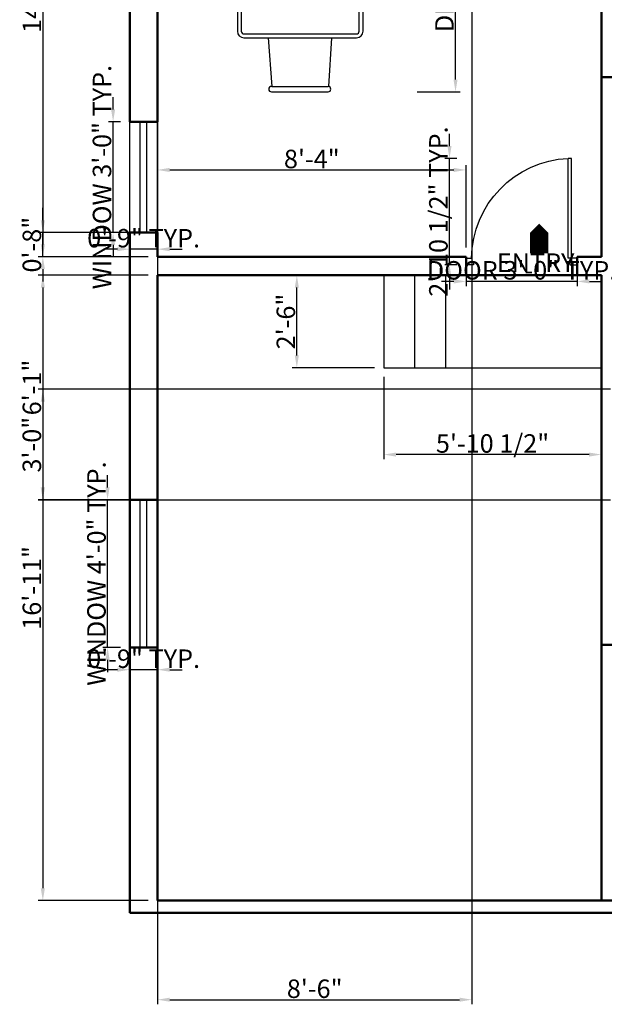
# Model space of a CAD drawing. Units: inches. Extents: x 749 to 1130, y 885 to 1490.
# Tile 1 of 5: x 754 to 944, y 885 to 1204. Entities that reach past the tile are written whole.
import ezdxf

# ---------------------------------------------------------------- set-up
doc = ezdxf.new("R2010")
doc.units = ezdxf.units.IN
doc.header["$MEASUREMENT"] = 0
doc.layers.add('a patt', color=33, linetype='Continuous')
for name, color, linetype, lineweight in [('A-ANNO-DIMS', 2, 'Continuous', 18), ('A-ANNO-SYMB', 3, 'Continuous', 18), ('A-AREA-IDEN', 7, 'Continuous', 25), ('A-DOOR', 2, 'Continuous', 25), ('A-FLOR-STRS', 7, 'Continuous', 25), ('A-FURN', 9, 'Continuous', 18), ('WALL', 7, 'Continuous', 50), ('WINDOW', 2, 'Continuous', 25)]:
    doc.layers.add(name, color=color, linetype=linetype, lineweight=lineweight)
doc.styles.get("Standard").update_dxf_attribs({"font": 'arial.ttf'})
doc.styles.add('YQ_DIM', font='SUPEROS.SHX', dxfattribs={"width": 0.8, "bigfont": 'HZDX.SHX'})
doc.dimstyles.new('yqi0', dxfattribs={"dimscale": 0, "dimtxt": 6, "dimasz": 4, "dimexe": 1.5, "dimexo": 3, "dimgap": 0.5, "dimtad": 1, "dimdsep": 46, "dimlunit": 4, "dimtxsty": 'Standard', "dimcen": 0, "dimclrd": 256, "dimclre": 256, "dimclrt": 7, "dimadec": 1, "dimazin": 2, "dimtfac": 1, "dimtix": 1, "dimtmove": 2, "dimatfit": 2, "dimfxl": 1, "dimtolj": 1, "dimtzin": 0, "dimarcsym": 0})

# ---------------------------------------------------------------- blocks, each defined once
blk = doc.blocks.new('WD_WIN4')
for p, q in [((-0.5, 0.5), (0.5, 0.5)), ((-0.5, 0.12), (0.5, 0.12)), ((-0.5, -0.12), (0.5, -0.12)), ((-0.5, -0.5), (0.5, -0.5))]:
    blk.add_line(p, q)
blk = doc.blocks.new('grdfg')
at = {"layer": 'a patt'}
for p, q in [((615.1, 1349.1), (612, 1348.9)), ((1015.8, 1349), (615, 1349)), ((615, 1348.9), (615, 1349)), ((1015.8, 1349.1), (1018.9, 1348.9)), ((1307.5, 1349.1), (1304.3, 1348.9)), ((1307.4, 1348.9), (1307.4, 1349)), ((1708.1, 1349), (1307.4, 1349)), ((1708.1, 1349.1), (1711.2, 1348.9)), ((589, 1028.2), (611.9, 1309.9)), ((609.3, 1310.2), (609.3, 1278.3)), ((1018.9, 1309.9), (611.8, 1309.9)), ((1041.8, 1028.2), (1018.9, 1310)), ((1281.4, 1028.2), (1304.2, 1309.9)), ((1711.2, 1309.9), (1304.2, 1309.9)), ((1734.1, 1028.2), (1711.3, 1310)), ((605.1, 1201.3), (603.1, 1201.3)), ((1297.4, 1201.3), (1295.4, 1201.3)), ((1850.7, 1028.2), (443.9, 1028.2)), ((1850.7, 1000.2), (443.9, 1000.2)), ((397.3, 981.6), (397.3, 174.8)), ((425.3, 981.6), (425.3, 174.8)), ((841.2, 969.6), (862.7, 969.6)), ((1560.1, 969.6), (1581.7, 969.6)), ((1869.3, 174.8), (1869.3, 981.6)), ((1897.3, 174.8), (1897.3, 981.6)), ((763.3, 888.1), (769.2, 888.1)), ((763.3, 878.9), (769.2, 878.9)), ((812.6, 857.1), (805.6, 857.1)), ((844.8, 869.7), (859.1, 869.7)), ((844.8, 858.9), (859.1, 858.9)), ((844.8, 851.7), (859.1, 851.7)), ((1482.3, 888.1), (1488.2, 888.1)), ((1482.3, 878.9), (1488.2, 878.9)), ((1531.6, 857.1), (1524.6, 857.1)), ((1563.7, 869.7), (1578.1, 869.7)), ((1563.7, 858.9), (1578.1, 858.9)), ((1563.7, 851.7), (1578.1, 851.7)), ((10, 784.9), (10, 377.8)), ((49.2, 781.8), (49, 784.9)), ((397.3, 807.5), (49.1, 781.7)), ((49.1, 781.7), (49.1, 381)), ((805.6, 844.8), (812.6, 844.8)), ((1524.6, 844.8), (1531.6, 844.8)), ((1897.3, 807.5), (2245.5, 781.7)), ((2245.4, 781.8), (2245.6, 784.9)), ((2245.5, 781.7), (2245.5, 381)), ((2284.6, 784.9), (2284.6, 377.8)), ((769.7, 504.8), (923, 351.5)), ((397.3, 355.1), (48.7, 375)), ((49.2, 381.1), (49, 378)), ((49, 381), (49.1, 381)), ((1897.3, 355.1), (2245.9, 375)), ((2245.4, 381.1), (2245.6, 378)), ((2245.6, 381), (2245.5, 381)), ((805.6, 311.6), (812.6, 311.6)), ((812.6, 299.3), (805.6, 299.3)), ((844.8, 304.7), (859.1, 304.7)), ((844.8, 297.5), (859.1, 297.5)), ((844.8, 286.7), (859.1, 286.7)), ((1524.6, 311.6), (1531.6, 311.6)), ((1531.6, 299.3), (1524.6, 299.3)), ((1563.7, 304.7), (1578.1, 304.7)), ((1563.7, 297.5), (1578.1, 297.5)), ((1563.7, 286.7), (1578.1, 286.7)), ((763.3, 277.5), (769.2, 277.5)), ((763.3, 268.3), (769.2, 268.3)), ((771, 235), (802.4, 235)), ((815.8, 235), (844.3, 235)), ((1482.3, 277.5), (1488.2, 277.5)), ((1482.3, 268.3), (1488.2, 268.3)), ((1490, 235), (1521.4, 235)), ((1534.8, 235), (1563.3, 235)), ((443.9, 156.2), (1850.7, 156.2)), ((841.2, 186.8), (862.7, 186.8)), ((1560.1, 186.8), (1581.7, 186.8)), ((443.9, 128.2), (1850.7, 128.2)), ((589, 128.2), (611.9, -153.5)), ((1041.8, 128.2), (1018.9, -153.6)), ((1281.4, 128.2), (1304.2, -153.5)), ((1734.1, 128.2), (1711.3, -153.6)), ((605.1, -44.9), (603.1, -44.9)), ((1027.7, -44.9), (1025.6, -44.9)), ((609.3, -122), (609.3, -153.8)), ((1018.9, -153.5), (611.8, -153.5)), ((615.1, -192.7), (612, -192.5)), ((615, -192.5), (615, -192.6)), ((1015.8, -192.6), (615, -192.6)), ((1015.8, -192.7), (1018.9, -192.5)), ((1711.2, -153.5), (1304.2, -153.5)), ((1307.5, -192.7), (1304.3, -192.5)), ((1307.4, -192.5), (1307.4, -192.6)), ((1708.1, -192.6), (1307.4, -192.6)), ((1708.1, -192.7), (1711.2, -192.5))]:
    blk.add_line(p, q, dxfattribs=at)
for points in [[(758.7, 967), (758.7, 954.7, -0.013852), (763.3, 888.1), (763.3, 878.9, -0.321801), (757.9, 871.5, 0.220637), (748.8, 856.4, 0.151079), (755.6, 820.3, 0.601255), (776.8, 820.3, 0.098298), (784.5, 845.7, 0.173345), (779.1, 866.9, 0.127575), (772.3, 873, -0.108886), (769.2, 878.9), (769.2, 888.1, -0.013852), (773.8, 954.7), (773.8, 967), (772.3, 982, 0.903848), (760.2, 982)], [(841.2, 985.7, 0.204141), (841.2, 969.6), (844.8, 914.2), (844.8, 869.7), (843, 862.5), (844.8, 858.9), (844.8, 851.7), (843, 846.6, -0.015744), (841.2, 721.5, 0.538165), (859.1, 721.5), (864.3, 846.6), (859.1, 851.7), (859.1, 858.9), (860.9, 862.5), (859.1, 869.7), (859.1, 914.2), (862.7, 969.6, 0.204141), (862.7, 985.7), (857.3, 987.5), (846.6, 987.5)], [(1477.7, 967), (1477.7, 954.7, -0.013852), (1482.3, 888.1), (1482.3, 878.9, -0.321801), (1476.9, 871.5, 0.220637), (1467.8, 856.4, 0.151079), (1474.6, 820.3, 0.601255), (1495.8, 820.3, 0.098298), (1503.5, 845.7, 0.173345), (1498.1, 866.9, 0.127575), (1491.2, 873, -0.108886), (1488.2, 878.9), (1488.2, 888.1, -0.013852), (1492.8, 954.7), (1492.8, 967), (1491.2, 982, 0.903848), (1479.2, 982)], [(1560.1, 985.7, 0.204141), (1560.1, 969.6), (1563.7, 914.2), (1563.7, 869.7), (1561.9, 862.5), (1563.7, 858.9), (1563.7, 851.7), (1561.9, 846.6, -0.015744), (1560.1, 721.5, 0.538165), (1578.1, 721.5), (1583.3, 846.6), (1578.1, 851.7), (1578.1, 858.9), (1579.9, 862.5), (1578.1, 869.7), (1578.1, 914.2), (1581.7, 969.6, 0.204141), (1581.7, 985.7), (1576.3, 987.5), (1565.5, 987.5)], [(841.2, 170.6, -0.204141), (841.2, 186.8), (844.8, 242.1), (844.8, 286.7), (843, 293.9), (844.8, 297.5), (844.8, 304.7), (843, 309.8, 0.015744), (841.2, 434.9, -0.538165), (859.1, 434.9), (864.3, 309.8), (859.1, 304.7), (859.1, 297.5), (860.9, 293.9), (859.1, 286.7), (859.1, 242.1), (862.7, 186.8, -0.204141), (862.7, 170.6), (857.3, 168.8), (846.6, 168.8)], [(1560.1, 170.6, -0.204141), (1560.1, 186.8), (1563.7, 242.1), (1563.7, 286.7), (1561.9, 293.9), (1563.7, 297.5), (1563.7, 304.7), (1561.9, 309.8, 0.015744), (1560.1, 434.9, -0.538165), (1578.1, 434.9), (1583.3, 309.8), (1578.1, 304.7), (1578.1, 297.5), (1579.9, 293.9), (1578.1, 286.7), (1578.1, 242.1), (1581.7, 186.8, -0.204141), (1581.7, 170.6), (1576.3, 168.8), (1565.5, 168.8)], [(758.7, 189.4), (758.7, 201.7, 0.013852), (763.3, 268.3), (763.3, 277.5, 0.321801), (757.9, 284.9, -0.220637), (748.8, 300, -0.151079), (755.6, 336.1, -0.601255), (776.8, 336.1, -0.098298), (784.5, 310.7, -0.173345), (779.1, 289.5, -0.127575), (772.3, 283.4, 0.108886), (769.2, 277.5), (769.2, 268.3, 0.013852), (773.8, 201.7), (773.8, 189.4), (772.3, 174.3, -0.903848), (760.2, 174.3)], [(1477.7, 189.4), (1477.7, 201.7, 0.013852), (1482.3, 268.3), (1482.3, 277.5, 0.321801), (1476.9, 284.9, -0.220637), (1467.8, 300, -0.151079), (1474.6, 336.1, -0.601255), (1495.8, 336.1, -0.098298), (1503.5, 310.7, -0.173345), (1498.1, 289.5, -0.127575), (1491.2, 283.4, 0.108886), (1488.2, 277.5), (1488.2, 268.3, 0.013852), (1492.8, 201.7), (1492.8, 189.4), (1491.2, 174.3, -0.903848), (1479.2, 174.3)]]:
    blk.add_lwpolyline(points, format="xyb", close=True, dxfattribs=at)
for points in [[(802, 981.9), (800.2, 964.2), (800.2, 950, -0.012883), (805.6, 857.1), (805.6, 844.8, -0.236068), (798.4, 834, 0.098033), (794.8, 814.4), (796.6, 759.1), (798.4, 759.1), (800.2, 814.4), (802, 814.4), (803.8, 759.1), (805.6, 759.1), (807.4, 816.2), (809.2, 818), (810.8, 816.2), (812.6, 759.1), (814.4, 759.1), (816.2, 814.4), (818, 814.4), (819.8, 759.1), (821.6, 759.1), (823.4, 814.4), (819.8, 834, -0.236068), (812.6, 844.8), (812.6, 857.1, -0.012883), (818, 950), (818, 964.2), (816.2, 981.9, 0.761905), (802, 981.9, 0.027392)], [(1521, 981.9), (1519.2, 964.2), (1519.2, 950, -0.012883), (1524.6, 857.1), (1524.6, 844.8, -0.236068), (1517.4, 834, 0.098033), (1513.8, 814.4), (1515.6, 759.1), (1517.4, 759.1), (1519.2, 814.4), (1521, 814.4), (1522.8, 759.1), (1524.6, 759.1), (1526.4, 816.2), (1528.2, 818), (1529.8, 816.2), (1531.6, 759.1), (1533.4, 759.1), (1535.2, 814.4), (1537, 814.4), (1538.8, 759.1), (1540.6, 759.1), (1542.4, 814.4), (1538.8, 834, -0.236068), (1531.6, 844.8), (1531.6, 857.1, -0.012883), (1537, 950), (1537, 964.2), (1535.2, 981.9, 0.761905), (1521, 981.9, 0.027392)], [(802, 174.5), (800.2, 192.2), (800.2, 206.4, 0.012883), (805.6, 299.3), (805.6, 311.6, 0.236068), (798.4, 322.4, -0.098033), (794.8, 342), (796.6, 397.3), (798.4, 397.3), (800.2, 342), (802, 342), (803.8, 397.3), (805.6, 397.3), (807.4, 340.2), (809.2, 338.4), (810.8, 340.2), (812.6, 397.3), (814.4, 397.3), (816.2, 342), (818, 342), (819.8, 397.3), (821.6, 397.3), (823.4, 342), (819.8, 322.4, 0.236068), (812.6, 311.6), (812.6, 299.3, 0.012883), (818, 206.4), (818, 192.2), (816.2, 174.5, -0.761905), (802, 174.5, -0.027392)], [(1521, 174.5), (1519.2, 192.2), (1519.2, 206.4, 0.012883), (1524.6, 299.3), (1524.6, 311.6, 0.236068), (1517.4, 322.4, -0.098033), (1513.8, 342), (1515.6, 397.3), (1517.4, 397.3), (1519.2, 342), (1521, 342), (1522.8, 397.3), (1524.6, 397.3), (1526.4, 340.2), (1528.2, 338.4), (1529.8, 340.2), (1531.6, 397.3), (1533.4, 397.3), (1535.2, 342), (1537, 342), (1538.8, 397.3), (1540.6, 397.3), (1542.4, 342), (1538.8, 322.4, 0.236068), (1531.6, 311.6), (1531.6, 299.3, 0.012883), (1537, 206.4), (1537, 192.2), (1535.2, 174.5, -0.761905), (1521, 174.5, -0.027392)]]:
    blk.add_lwpolyline(points, format="xyb", dxfattribs=at)
for centre, radius, start, end in [((612.9, 1329.4), 19.5, 92.49117, 267.90507), ((1018, 1329.4), 19.5, 272.09493, 87.50883), ((1305.2, 1329.4), 19.5, 92.49117, 267.90507), ((1710.4, 1329.4), 19.5, 272.09493, 87.50883), ((443.9, 981.6), 46.6, 90, 180), ((443.9, 981.6), 18.7, 90, 180), ((1850.7, 981.6), 46.6, 0, 90), ((1850.7, 981.6), 18.7, 0, 90), ((805.7, 784), 122.1, 110.56901, 64.06758), ((805.7, 784), 88.4, 130.41773, 52.83265), ((805.7, 784), 122.1, 91.10258, 107.11677), ((805.7, 784), 88.4, 90.42812, 108.06348), ((805.7, 784), 88.4, 64.83762, 85.19102), ((805.7, 784), 122.1, 71.3681, 85.72946), ((1524.7, 784), 122.1, 110.56901, 64.06758), ((1524.7, 784), 88.4, 130.41773, 52.83265), ((1524.7, 784), 122.1, 91.10258, 107.11677), ((1524.7, 784), 88.4, 90.42812, 108.06348), ((1524.7, 784), 88.4, 64.83762, 85.19102), ((1524.7, 784), 122.1, 71.3681, 85.72946), ((29.5, 784), 19.5, 2.49118, 177.90507), ((2265.1, 784), 19.5, 2.09493, 177.50882), ((805.7, 372.4), 122.1, 295.93242, 249.43099), ((1524.7, 372.4), 122.1, 295.93242, 249.43099), ((805.7, 372.4), 88.4, 307.16735, 229.58227), ((1524.7, 372.4), 88.4, 307.16735, 229.58227), ((29.5, 378.8), 19.5, 182.09493, 357.50882), ((2265.1, 378.8), 19.5, 182.49118, 357.90507), ((805.7, 372.4), 88.4, 251.93652, 269.57188), ((805.7, 372.4), 88.4, 274.80898, 295.16238), ((1524.7, 372.4), 88.4, 251.93652, 269.57188), ((1524.7, 372.4), 88.4, 274.80898, 295.16238), ((805.7, 372.4), 122.1, 252.88323, 268.89742), ((805.7, 372.4), 122.1, 274.27054, 288.6319), ((1524.7, 372.4), 122.1, 252.88323, 268.89742), ((1524.7, 372.4), 122.1, 274.27054, 288.6319), ((443.9, 174.8), 46.6, 180, 270), ((443.9, 174.8), 18.7, 180, 270), ((1850.7, 174.8), 46.6, 270, 0), ((1850.7, 174.8), 18.7, 270, 0), ((612.9, -173), 19.5, 92.09493, 267.50883), ((1018, -173), 19.5, 272.49117, 87.90507), ((1305.2, -173), 19.5, 92.09493, 267.50883), ((1710.4, -173), 19.5, 272.49117, 87.90507)]:
    blk.add_arc(centre, radius, start, end, dxfattribs=at)
blk = doc.blocks.new('DR_D01')
for p, q in [((-0.45, 0.93), (-0.42, 0.93)), ((-0.45, 0.03), (-0.45, 0.93)), ((-0.42, 0.03), (-0.42, 0.93)), ((-0.5, 0.03), (-0.42, 0.03)), ((-0.5, 0.03), (-0.5, -0.03)), ((-0.45, 0.03), (-0.45, 0)), ((-0.45, 0), (-0.435, 0)), ((-0.435, 0), (-0.435, -0.03)), ((0.435, 0), (0.435, -0.03)), ((0.45, 0), (0.435, 0)), ((0.45, 0.03), (0.45, 0)), ((0.5, 0.03), (0.45, 0.03)), ((0.5, -0.03), (0.5, 0.03)), ((-0.435, -0.03), (-0.5, -0.03)), ((0.435, -0.03), (0.5, -0.03))]:
    blk.add_line(p, q)
blk.add_arc((-0.4602, 0.0206), 0.9103, 0.59152, 87.46644)
blk = doc.blocks.new('*D11')
at = {"layer": 'A-ANNO-DIMS', "lineweight": -2, "transparency": 16777216}
for p, q in [((782.87, 1052.6), (782.87, 1056.6)), ((787.07, 1048.6), (781.37, 1048.6)), ((782.87, 1000.6), (782.87, 1048.6)), ((787.07, 1000.6), (781.37, 1000.6)), ((782.87, 996.6), (782.87, 992.6))]:
    blk.add_line(p, q, dxfattribs=at)
at = {"layer": 'A-ANNO-DIMS', "transparency": 16777216}
for points in [[(782.2, 1052.6), (783.54, 1052.6), (782.87, 1048.6)], [(782.2, 996.6), (783.54, 996.6), (782.87, 1000.6)]]:
    blk.add_solid(points, dxfattribs=at)
at = {"layer": 'Defpoints', "color": 0, "transparency": 16777216}
for p in [(782.87, 1048.6), (790.07, 1048.6), (790.07, 1000.6)]:
    blk.add_point(p, dxfattribs=at)
at = {"layer": 'A-ANNO-DIMS', "color": 7, "transparency": 16777216, "insert": (779.27, 1024.6), "char_height": 6, "attachment_point": 5, "rotation": 90}
blk.add_mtext('\\A1;WINDOW 4\'-0" TYP.', dxfattribs=at)
blk = doc.blocks.new('*D12')
at = {"layer": 'A-ANNO-DIMS', "lineweight": -2, "transparency": 16777216}
for p, q in [((790.07, 997.6), (790.07, 991.9)), ((799.07, 997.6), (799.07, 991.9)), ((786.07, 993.4), (782.07, 993.4)), ((799.07, 993.4), (790.07, 993.4)), ((803.07, 993.4), (807.07, 993.4))]:
    blk.add_line(p, q, dxfattribs=at)
at = {"layer": 'A-ANNO-DIMS', "transparency": 16777216}
for points in [[(786.07, 994.07), (786.07, 992.74), (790.07, 993.4)], [(803.07, 994.07), (803.07, 992.74), (799.07, 993.4)]]:
    blk.add_solid(points, dxfattribs=at)
at = {"layer": 'Defpoints', "color": 0, "transparency": 16777216}
for p in [(790.07, 1000.6), (799.07, 1000.6), (790.07, 993.4)]:
    blk.add_point(p, dxfattribs=at)
at = {"layer": 'A-ANNO-DIMS', "color": 7, "transparency": 16777216, "insert": (794.57, 996.97), "char_height": 6, "attachment_point": 5}
blk.add_mtext('\\A1;0\'-9" TYP.', dxfattribs=at)
blk = doc.blocks.new('*D13')
at = {"layer": 'A-ANNO-DIMS', "lineweight": -2, "transparency": 16777216}
for p, q in [((784.67, 1175.33), (784.67, 1179.33)), ((787.07, 1171.33), (783.17, 1171.33)), ((784.67, 1135.33), (784.67, 1171.33)), ((787.07, 1135.33), (783.17, 1135.33)), ((784.67, 1131.33), (784.67, 1127.33))]:
    blk.add_line(p, q, dxfattribs=at)
at = {"layer": 'A-ANNO-DIMS', "transparency": 16777216}
for points in [[(784, 1175.33), (785.34, 1175.33), (784.67, 1171.33)], [(784, 1131.33), (785.34, 1131.33), (784.67, 1135.33)]]:
    blk.add_solid(points, dxfattribs=at)
at = {"layer": 'Defpoints', "color": 0, "transparency": 16777216}
for p in [(784.67, 1171.33), (790.07, 1171.33), (790.07, 1135.33)]:
    blk.add_point(p, dxfattribs=at)
at = {"layer": 'A-ANNO-DIMS', "color": 7, "transparency": 16777216, "insert": (781.06, 1153.33), "char_height": 6, "attachment_point": 5, "rotation": 90}
blk.add_mtext('\\A1;WINDOW 3\'-0" TYP.', dxfattribs=at)
blk = doc.blocks.new('*D14')
at = {"layer": 'A-ANNO-DIMS', "lineweight": -2, "transparency": 16777216}
for p, q in [((790.07, 1132.33), (790.07, 1128.43)), ((799.07, 1132.33), (799.07, 1128.43)), ((786.07, 1129.93), (782.07, 1129.93)), ((799.07, 1129.93), (790.07, 1129.93)), ((803.07, 1129.93), (807.07, 1129.93))]:
    blk.add_line(p, q, dxfattribs=at)
at = {"layer": 'A-ANNO-DIMS', "transparency": 16777216}
for points in [[(786.07, 1130.6), (786.07, 1129.27), (790.07, 1129.93)], [(803.07, 1130.6), (803.07, 1129.27), (799.07, 1129.93)]]:
    blk.add_solid(points, dxfattribs=at)
at = {"layer": 'Defpoints', "color": 0, "transparency": 16777216}
for p in [(790.07, 1135.33), (799.07, 1135.33), (790.07, 1129.93)]:
    blk.add_point(p, dxfattribs=at)
at = {"layer": 'A-ANNO-DIMS', "color": 7, "transparency": 16777216, "insert": (794.57, 1133.5), "char_height": 6, "attachment_point": 5}
blk.add_mtext('\\A1;0\'-9" TYP.', dxfattribs=at)
blk = doc.blocks.new('*D17')
at = {"layer": 'A-ANNO-DIMS', "lineweight": -2, "transparency": 16777216}
for p, q in [((895.2, 1119.47), (891.2, 1119.47)), ((899.2, 1121.87), (899.2, 1117.97)), ((935.2, 1119.47), (899.2, 1119.47)), ((935.2, 1121.87), (935.2, 1117.97)), ((939.2, 1119.47), (943.2, 1119.47))]:
    blk.add_line(p, q, dxfattribs=at)
at = {"layer": 'A-ANNO-DIMS', "transparency": 16777216}
for points in [[(895.2, 1120.13), (895.2, 1118.8), (899.2, 1119.47)], [(939.2, 1120.13), (939.2, 1118.8), (935.2, 1119.47)]]:
    blk.add_solid(points, dxfattribs=at)
at = {"layer": 'Defpoints', "color": 0, "transparency": 16777216}
for p in [(899.2, 1124.87), (935.2, 1124.87), (899.2, 1119.47)]:
    blk.add_point(p, dxfattribs=at)
at = {"layer": 'A-ANNO-DIMS', "color": 7, "transparency": 16777216, "insert": (917.2, 1123.07), "char_height": 6, "attachment_point": 5}
blk.add_mtext('\\A1;DOOR 3\'-0" TYP.', dxfattribs=at)
blk = doc.blocks.new('*D18')
at = {"layer": 'A-ANNO-DIMS', "lineweight": -2, "transparency": 16777216}
for p, q in [((893.8, 1163.43), (893.8, 1167.43)), ((896.2, 1159.43), (892.3, 1159.43)), ((893.8, 1124.87), (893.8, 1159.43)), ((896.2, 1124.87), (892.3, 1124.87)), ((893.8, 1120.87), (893.8, 1116.87))]:
    blk.add_line(p, q, dxfattribs=at)
at = {"layer": 'A-ANNO-DIMS', "transparency": 16777216}
for points in [[(893.14, 1163.43), (894.47, 1163.43), (893.8, 1159.43)], [(893.14, 1120.87), (894.47, 1120.87), (893.8, 1124.87)]]:
    blk.add_solid(points, dxfattribs=at)
at = {"layer": 'Defpoints', "color": 0, "transparency": 16777216}
for p in [(893.8, 1159.43), (899.2, 1159.43), (899.2, 1124.87)]:
    blk.add_point(p, dxfattribs=at)
at = {"layer": 'A-ANNO-DIMS', "color": 7, "transparency": 16777216, "insert": (890.2, 1142.15), "char_height": 6, "attachment_point": 5, "rotation": 90}
blk.add_mtext('\\A1;2\'-10 1/2" TYP.', dxfattribs=at)
blk = doc.blocks.new('*D29')
at = {"layer": 'A-ANNO-DIMS', "lineweight": -2, "transparency": 16777216}
for p, q in [((883.31, 1284.07), (897.27, 1284.07)), ((895.77, 1185.01), (895.77, 1280.07)), ((883.31, 1181.01), (897.27, 1181.01))]:
    blk.add_line(p, q, dxfattribs=at)
at = {"layer": 'A-ANNO-DIMS', "transparency": 16777216}
for points in [[(895.1, 1280.07), (896.43, 1280.07), (895.77, 1284.07)], [(895.1, 1185.01), (896.43, 1185.01), (895.77, 1181.01)]]:
    blk.add_solid(points, dxfattribs=at)
at = {"layer": 'Defpoints', "color": 0, "transparency": 16777216}
for p in [(880.31, 1284.07), (895.77, 1284.07), (880.31, 1181.01)]:
    blk.add_point(p, dxfattribs=at)
at = {"layer": 'A-ANNO-DIMS', "color": 7, "transparency": 16777216, "insert": (892.16, 1232.54), "char_height": 6, "attachment_point": 5, "rotation": 90}
blk.add_mtext('\\A1;DINING SET 8\'-7"', dxfattribs=at)
blk = doc.blocks.new('*D34')
at = {"layer": 'A-ANNO-DIMS', "lineweight": -2, "transparency": 16777216}
for p, q in [((796.07, 1295.46), (760.37, 1295.46)), ((761.87, 1291.46), (761.87, 1131.46)), ((796.07, 1127.46), (760.37, 1127.46))]:
    blk.add_line(p, q, dxfattribs=at)
at = {"layer": 'A-ANNO-DIMS', "transparency": 16777216}
for points in [[(761.2, 1291.46), (762.54, 1291.46), (761.87, 1295.46)], [(761.2, 1131.46), (762.54, 1131.46), (761.87, 1127.46)]]:
    blk.add_solid(points, dxfattribs=at)
at = {"layer": 'Defpoints', "color": 0, "transparency": 16777216}
for p in [(799.07, 1295.46), (761.87, 1127.46), (799.07, 1127.46)]:
    blk.add_point(p, dxfattribs=at)
at = {"layer": 'A-ANNO-DIMS', "color": 7, "transparency": 16777216, "insert": (758.31, 1211.46), "char_height": 6, "attachment_point": 5, "rotation": 90}
blk.add_mtext('\\A1;14\'-0"', dxfattribs=at)
blk = doc.blocks.new('*D35')
at = {"layer": 'A-ANNO-DIMS', "lineweight": -2, "transparency": 16777216}
for p, q in [((796.07, 1121.46), (760.37, 1121.46)), ((761.87, 1117.46), (761.87, 922.46)), ((796.07, 918.46), (760.37, 918.46))]:
    blk.add_line(p, q, dxfattribs=at)
at = {"layer": 'A-ANNO-DIMS', "transparency": 16777216}
for points in [[(761.2, 1117.46), (762.54, 1117.46), (761.87, 1121.46)], [(761.2, 922.46), (762.54, 922.46), (761.87, 918.46)]]:
    blk.add_solid(points, dxfattribs=at)
at = {"layer": 'Defpoints', "color": 0, "transparency": 16777216}
for p in [(799.07, 1121.46), (761.87, 918.46), (799.07, 918.46)]:
    blk.add_point(p, dxfattribs=at)
at = {"layer": 'A-ANNO-DIMS', "color": 7, "transparency": 16777216, "insert": (758.31, 1019.96), "char_height": 6, "attachment_point": 5, "rotation": 90}
blk.add_mtext('\\A1;16\'-11"', dxfattribs=at)
blk = doc.blocks.new('*D41')
at = {"layer": 'A-ANNO-DIMS', "lineweight": -2, "transparency": 16777216}
for p, q in [((799.07, 1298.46), (799.07, 884.76)), ((901.07, 1298.46), (901.07, 884.76)), ((803.07, 886.26), (897.07, 886.26))]:
    blk.add_line(p, q, dxfattribs=at)
at = {"layer": 'A-ANNO-DIMS', "transparency": 16777216}
for points in [[(803.07, 886.93), (803.07, 885.59), (799.07, 886.26)], [(897.07, 886.93), (897.07, 885.59), (901.07, 886.26)]]:
    blk.add_solid(points, dxfattribs=at)
at = {"layer": 'Defpoints', "color": 0, "transparency": 16777216}
for p in [(799.07, 1301.46), (901.07, 1301.46), (901.07, 886.26)]:
    blk.add_point(p, dxfattribs=at)
at = {"layer": 'A-ANNO-DIMS', "color": 7, "transparency": 16777216, "insert": (850.07, 889.82), "char_height": 6, "attachment_point": 5}
blk.add_mtext('\\A1;8\'-6"', dxfattribs=at)
blk = doc.blocks.new('*D47')
at = {"layer": 'A-ANNO-DIMS', "lineweight": -2, "transparency": 16777216}
for p, q in [((949.07, 1087.46), (949.07, 1484.16)), ((959.07, 1087.46), (959.07, 1484.16)), ((945.07, 1482.66), (941.07, 1482.66)), ((949.07, 1482.66), (959.07, 1482.66)), ((963.07, 1482.66), (967.07, 1482.66))]:
    blk.add_line(p, q, dxfattribs=at)
at = {"layer": 'A-ANNO-DIMS', "transparency": 16777216}
for points in [[(945.07, 1483.33), (945.07, 1481.99), (949.07, 1482.66)], [(963.07, 1483.33), (963.07, 1481.99), (959.07, 1482.66)]]:
    blk.add_solid(points, dxfattribs=at)
at = {"layer": 'Defpoints', "color": 0, "transparency": 16777216}
for p in [(959.07, 1482.66), (949.07, 1084.46), (959.07, 1084.46)]:
    blk.add_point(p, dxfattribs=at)
at = {"layer": 'A-ANNO-DIMS', "color": 7, "transparency": 16777216, "insert": (954.07, 1486.22), "char_height": 6, "attachment_point": 5}
blk.add_mtext('\\A1;0\'-10"', dxfattribs=at)
blk = doc.blocks.new('*D49')
at = {"layer": 'A-ANNO-DIMS', "lineweight": -2, "transparency": 16777216}
for p, q in [((946.07, 1084.46), (760.37, 1084.46)), ((761.87, 1080.46), (761.87, 1052.46)), ((946.07, 1048.46), (760.37, 1048.46))]:
    blk.add_line(p, q, dxfattribs=at)
at = {"layer": 'A-ANNO-DIMS', "transparency": 16777216}
for points in [[(761.2, 1080.46), (762.54, 1080.46), (761.87, 1084.46)], [(761.2, 1052.46), (762.54, 1052.46), (761.87, 1048.46)]]:
    blk.add_solid(points, dxfattribs=at)
at = {"layer": 'Defpoints', "color": 0, "transparency": 16777216}
for p in [(949.07, 1084.46), (761.87, 1048.46), (949.07, 1048.46)]:
    blk.add_point(p, dxfattribs=at)
at = {"layer": 'A-ANNO-DIMS', "color": 7, "transparency": 16777216, "insert": (758.3, 1066.46), "char_height": 6, "attachment_point": 5, "rotation": 90}
blk.add_mtext('\\A1;3\'-0"', dxfattribs=at)
blk = doc.blocks.new('*D55')
at = {"layer": 'A-ANNO-DIMS', "lineweight": -2, "transparency": 16777216}
for p, q in [((761.87, 1139.33), (761.87, 1143.33)), ((796.07, 1135.33), (760.37, 1135.33)), ((761.87, 1127.46), (761.87, 1135.33)), ((796.07, 1127.46), (760.37, 1127.46)), ((761.87, 1123.46), (761.87, 1119.46))]:
    blk.add_line(p, q, dxfattribs=at)
at = {"layer": 'A-ANNO-DIMS', "transparency": 16777216}
for points in [[(761.2, 1139.33), (762.54, 1139.33), (761.87, 1135.33)], [(761.2, 1123.46), (762.54, 1123.46), (761.87, 1127.46)]]:
    blk.add_solid(points, dxfattribs=at)
at = {"layer": 'Defpoints', "color": 0, "transparency": 16777216}
for p in [(761.87, 1135.33), (799.07, 1135.33), (799.07, 1127.46)]:
    blk.add_point(p, dxfattribs=at)
at = {"layer": 'A-ANNO-DIMS', "color": 7, "transparency": 16777216, "insert": (758.31, 1131.4), "char_height": 6, "attachment_point": 5, "rotation": 90}
blk.add_mtext('\\A1;0\'-8"', dxfattribs=at)
blk = doc.blocks.new('*D56')
at = {"layer": 'A-ANNO-DIMS', "lineweight": -2, "transparency": 16777216}
for p, q in [((796.07, 1121.46), (760.37, 1121.46)), ((761.87, 1117.46), (761.87, 1052.6)), ((796.07, 1048.6), (760.37, 1048.6))]:
    blk.add_line(p, q, dxfattribs=at)
at = {"layer": 'A-ANNO-DIMS', "transparency": 16777216}
for points in [[(761.2, 1117.46), (762.54, 1117.46), (761.87, 1121.46)], [(761.2, 1052.6), (762.54, 1052.6), (761.87, 1048.6)]]:
    blk.add_solid(points, dxfattribs=at)
at = {"layer": 'Defpoints', "color": 0, "transparency": 16777216}
for p in [(799.07, 1121.46), (761.87, 1048.6), (799.07, 1048.6)]:
    blk.add_point(p, dxfattribs=at)
at = {"layer": 'A-ANNO-DIMS', "color": 7, "transparency": 16777216, "insert": (758.31, 1085.03), "char_height": 6, "attachment_point": 5, "rotation": 90}
blk.add_mtext('\\A1;6\'-1"', dxfattribs=at)
blk = doc.blocks.new('*D61')
at = {"layer": 'A-ANNO-DIMS', "lineweight": -2, "transparency": 16777216}
for p, q in [((799.07, 1130.46), (799.07, 1157.16)), ((803.07, 1155.66), (895.2, 1155.66)), ((899.2, 1130.46), (899.2, 1157.16))]:
    blk.add_line(p, q, dxfattribs=at)
at = {"layer": 'A-ANNO-DIMS', "transparency": 16777216}
for points in [[(803.07, 1156.33), (803.07, 1154.99), (799.07, 1155.66)], [(895.2, 1156.33), (895.2, 1154.99), (899.2, 1155.66)]]:
    blk.add_solid(points, dxfattribs=at)
at = {"layer": 'Defpoints', "color": 0, "transparency": 16777216}
for p in [(899.2, 1155.66), (799.07, 1127.46), (899.2, 1127.46)]:
    blk.add_point(p, dxfattribs=at)
at = {"layer": 'A-ANNO-DIMS', "color": 7, "transparency": 16777216, "insert": (849.13, 1159.22), "char_height": 6, "attachment_point": 5}
blk.add_mtext('\\A1;8\'-4"', dxfattribs=at)
blk = doc.blocks.new('*D62')
at = {"layer": 'A-ANNO-DIMS', "lineweight": -2, "transparency": 16777216}
for p, q in [((872.48, 1088.45), (872.48, 1061.75)), ((943.07, 1088.45), (943.07, 1061.75)), ((939.07, 1063.25), (876.48, 1063.25))]:
    blk.add_line(p, q, dxfattribs=at)
at = {"layer": 'A-ANNO-DIMS', "transparency": 16777216}
for points in [[(876.48, 1063.91), (876.48, 1062.58), (872.48, 1063.25)], [(939.07, 1063.91), (939.07, 1062.58), (943.07, 1063.25)]]:
    blk.add_solid(points, dxfattribs=at)
at = {"layer": 'Defpoints', "color": 0, "transparency": 16777216}
for p in [(872.48, 1091.45), (943.07, 1091.45), (872.48, 1063.25)]:
    blk.add_point(p, dxfattribs=at)
at = {"layer": 'A-ANNO-DIMS', "color": 7, "transparency": 16777216, "insert": (907.77, 1066.85), "char_height": 6, "attachment_point": 5}
blk.add_mtext('\\A1;5\'-10 1/2"', dxfattribs=at)
blk = doc.blocks.new('*D63')
at = {"layer": 'A-ANNO-DIMS', "lineweight": -2, "transparency": 16777216}
for p, q in [((869.48, 1121.45), (842.78, 1121.45)), ((844.28, 1095.45), (844.28, 1117.45)), ((869.48, 1091.45), (842.78, 1091.45))]:
    blk.add_line(p, q, dxfattribs=at)
at = {"layer": 'A-ANNO-DIMS', "transparency": 16777216}
for points in [[(843.61, 1117.45), (844.94, 1117.45), (844.28, 1121.45)], [(843.61, 1095.45), (844.94, 1095.45), (844.28, 1091.45)]]:
    blk.add_solid(points, dxfattribs=at)
at = {"layer": 'Defpoints', "color": 0, "transparency": 16777216}
for p in [(844.28, 1121.45), (872.48, 1121.45), (872.48, 1091.45)]:
    blk.add_point(p, dxfattribs=at)
at = {"layer": 'A-ANNO-DIMS', "color": 7, "transparency": 16777216, "insert": (840.71, 1106.45), "char_height": 6, "attachment_point": 5, "rotation": 90}
blk.add_mtext('\\A1;2\'-6"', dxfattribs=at)

msp = doc.modelspace()

# ---------------------------------------------------------------- linework, layer by layer
at = {"layer": 'A-ANNO-SYMB'}
msp.add_lwpolyline([(922.902, 1138.223, 0, 12, 0), (922.902, 1132.223, 6, 6, 0), (922.902, 1128.623, 6, 6, 0)], format="xyseb", dxfattribs=at)
at = {"layer": 'A-FLOR-STRS'}
for p, q in [((872.478, 1121.445), (872.478, 1091.445)), ((882.478, 1121.445), (882.478, 1091.445)), ((892.478, 1121.445), (892.478, 1091.445)), ((872.478, 1091.445), (943.07, 1091.445))]:
    msp.add_line(p, q, dxfattribs=at)
at = {"layer": 'WALL'}
for p, q in [((790.07, 1171.334), (790.07, 1251.586)), ((799.07, 1171.334), (799.07, 1251.586)), ((943.07, 1171.334), (943.07, 1221.834)), ((943.07, 1127.46), (943.07, 1185.834)), ((943.07, 1185.834), (949.07, 1185.834)), ((799.07, 1171.334), (790.07, 1171.334)), ((790.07, 914.46), (790.07, 1135.334)), ((799.07, 1135.334), (790.07, 1135.334)), ((799.07, 1127.46), (799.07, 1135.334)), ((799.07, 1127.46), (899.196, 1127.46)), ((899.196, 1127.46), (899.196, 1121.46)), ((899.202, 1127.025), (899.202, 1121.445)), ((935.196, 1127.46), (943.07, 1127.46)), ((935.196, 1127.46), (935.196, 1121.46)), ((935.202, 1127.46), (935.202, 1121.445)), ((799.07, 1121.46), (935.196, 1121.46)), ((799.07, 1121.46), (799.07, 918.46)), ((935.196, 1121.46), (943.07, 1121.46)), ((943.07, 1083.46), (943.07, 1121.46)), ((943.07, 1083.46), (943.07, 918.46)), ((799.07, 1048.602), (790.07, 1048.602)), ((943.07, 1001.46), (1086.07, 1001.46)), ((799.07, 1000.602), (790.07, 1000.602)), ((799.07, 918.46), (943.07, 918.46)), ((943.07, 918.46), (1086.07, 918.46)), ((790.07, 914.46), (1090.07, 914.46))]:
    msp.add_line(p, q, dxfattribs=at)

# ---------------------------------------------------------------- block references
at = {"layer": 'A-DOOR', "xscale": 36, "yscale": -36, "zscale": 36, "rotation": 180}
msp.add_blockref('DR_D01', (917.202, 1125.945), dxfattribs=at)
at = {"layer": 'A-FURN', "xscale": 0.0453086432222982, "yscale": 0.0453086432222982, "zscale": 0.0453086432222982, "rotation": 90}
msp.add_blockref('grdfg', (871.578, 1180.561), dxfattribs=at)
at = {"layer": 'WINDOW'}
for p, xscale, yscale, zscale, rotation in [((794.57, 1153.334), 36, 9.000000000000341, 36, 89.99999999999982), ((794.57, 1024.602), 48, 9, 48, 90)]:
    msp.add_blockref('WD_WIN4', p, dxfattribs=dict(at, xscale=xscale, yscale=yscale, zscale=zscale, rotation=rotation))

# ---------------------------------------------------------------- texts
at = {"layer": 'A-AREA-IDEN', "insert": (910.097, 1128.576), "char_height": 13.77953, "width": 23.35911, "attachment_point": 1, "style": 'YQ_DIM'}
msp.add_mtext('\\pxqc;{\\H0.43543x;ENTRY}', dxfattribs=at)

# ---------------------------------------------------------------- dimensions: what is measured, and where the dimension line sits
at = {"layer": 'A-ANNO-DIMS'}
for base, p1, p2, picture, middle in [((959.07, 1482.66), (949.07, 1084.46), (959.07, 1084.46), '*D47', (954.07, 1486.224)), ((901.07, 886.26), (799.07, 1301.46), (901.07, 1301.46), '*D41', (850.07, 889.824)), ((899.196, 1155.66), (799.07, 1127.46), (899.196, 1127.46), '*D61', (849.133, 1159.224))]:
    dim = msp.add_linear_dim(base=base, p1=p1, p2=p2, dimstyle='yqi0', override={"dimscale": 1, "dimdec": 1, "dimzin": 1, "dimfrac": 2}, dxfattribs=at)
    dim.commit()
    dim.dimension.update_dxf_attribs({"geometry": picture, "text_midpoint": middle})
for base, p1, p2, angle, picture, middle in [((761.87, 1127.46), (799.07, 1295.46), (799.07, 1127.46), 90, '*D34', (758.306, 1211.46)), ((761.87, 1135.334), (799.07, 1127.46), (799.07, 1135.334), 90, '*D55', (758.306, 1131.397)), ((761.87, 918.46), (799.07, 1121.46), (799.07, 918.46), 90, '*D35', (758.306, 1019.96)), ((761.87, 1048.602), (799.07, 1121.46), (799.07, 1048.602), 90, '*D56', (758.306, 1085.031)), ((844.278, 1121.445), (872.478, 1091.445), (872.478, 1121.445), 90, '*D63', (840.714, 1106.445)), ((872.478, 1063.245), (943.07, 1091.445), (872.478, 1091.445), 180, '*D62', (907.774, 1066.848)), ((761.87, 1048.46), (949.07, 1084.46), (949.07, 1048.46), 90, '*D49', (758.304, 1066.46))]:
    dim = msp.add_linear_dim(base=base, p1=p1, p2=p2, angle=angle, dimstyle='yqi0', override={"dimscale": 1, "dimdec": 1, "dimzin": 1, "dimfrac": 2}, dxfattribs=at)
    dim.commit()
    dim.dimension.update_dxf_attribs({"geometry": picture, "text_midpoint": middle})
for base, p1, p2, angle, text, picture, middle in [((895.767, 1284.074), (880.308, 1181.013), (880.308, 1284.074), 90, 'DINING SET <>', '*D29', (892.165, 1232.544)), ((784.67, 1171.334), (790.07, 1135.334), (790.07, 1171.334), 90, 'WINDOW <> TYP.', '*D13', (781.064, 1153.334)), ((893.802, 1159.425), (899.202, 1124.865), (899.202, 1159.425), 90, '<> TYP.', '*D18', (890.2, 1142.145)), ((790.07, 1129.934), (799.07, 1135.334), (790.07, 1135.334), 180, '<> TYP.', '*D14', (794.57, 1133.498)), ((899.202, 1119.465), (935.202, 1124.865), (899.202, 1124.865), 180, 'DOOR <> TYP.', '*D17', (917.202, 1123.072)), ((782.87, 1048.602), (790.07, 1000.602), (790.07, 1048.602), 90, 'WINDOW <> TYP.', '*D11', (779.266, 1024.602)), ((790.07, 993.402), (799.07, 1000.602), (790.07, 1000.602), 180, '<> TYP.', '*D12', (794.57, 996.965))]:
    dim = msp.add_linear_dim(base=base, p1=p1, p2=p2, angle=angle, text=text, dimstyle='yqi0', override={"dimscale": 1, "dimdec": 1, "dimzin": 1, "dimfrac": 2}, dxfattribs=at)
    dim.commit()
    dim.dimension.update_dxf_attribs({"geometry": picture, "text_midpoint": middle})

doc.saveas('drawing.dxf')
